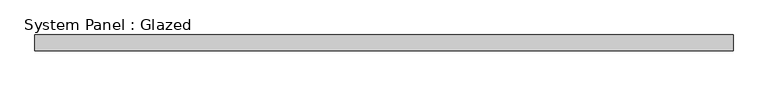
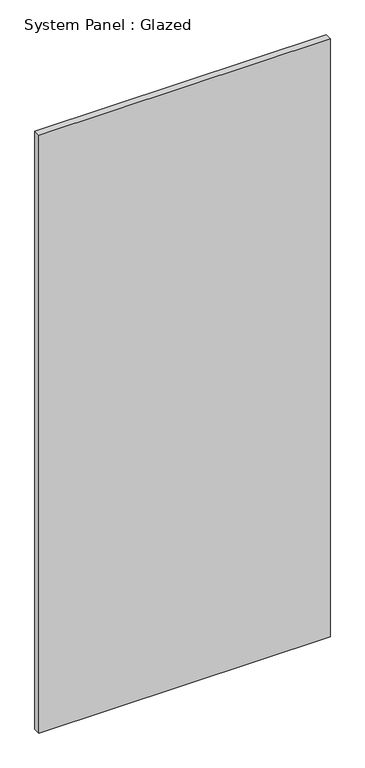
"""IFC4 building model written with IfcOpenShell, lengths in millimetres: plate geometry, System Panel : Glazed."""

from ifc_helpers import new_model, si_unit, origin, origin_with_axes, place, context, project, spatial, polyline, outline, extrude, source, transform, mapped, element, save


def system_panel_glazed_0c115810(model_context):
    return source(origin(), model_context, "Body", "SweptSolid", [
        extrude(outline(polyline([(561.975, 19.05), (-561.975, 19.05), (-561.975, 44.45), (561.975, 44.45), (561.975, 19.05)])), origin_with_axes(), (0.0, 0.0, 1.0), 2438.4),
    ])


if __name__ == "__main__":
    model = new_model("IFC4")
    model_context = context("Model", 3, world=origin())
    ifc_project = project(units=[si_unit("LENGTHUNIT", "METRE", prefix="MILLI")], contexts=[model_context])
    site = spatial("IfcSite", under=ifc_project)
    building = spatial("IfcBuilding", under=site)
    placement = place(None, origin())
    system_panel_glazed_shape = system_panel_glazed_0c115810(model_context)
    element("IfcPlate", 1, ObjectType="System Panel : Glazed", at=placement, inside=building, context=model_context, shape_type="MappedRepresentation", body=[
        mapped(system_panel_glazed_shape, transform((0.0, 0.0, 0.0), x_axis=(1.0, 0.0, 0.0), y_axis=(0.0, 1.0, 0.0), z_axis=(0.0, 0.0, 1.0))),
    ])
    save(model, "model.ifc")

# Revit data of these elements
# Type "System Panel : Glazed"
#   Construction Type Id = "GSP4R"
#   Analytic Construction = "1/8 in Pilkington single glazing"
#   Visual Light Transmittance = 0.9
#   Solar Heat Gain Coefficient = 0.86
#   Heat Transfer Coefficient (U) = 1.18115 BTU/(h·ft²·°F)
# Element 1 (IfcPlate, "System Panel : Glazed")
#   Materials on its faces: "Glass"
# Materials
#   "Glass": class "Glass", colour RGB 0 128 192, transparency 0.75, Description = "Soda Lime Glass", Cost = 0
